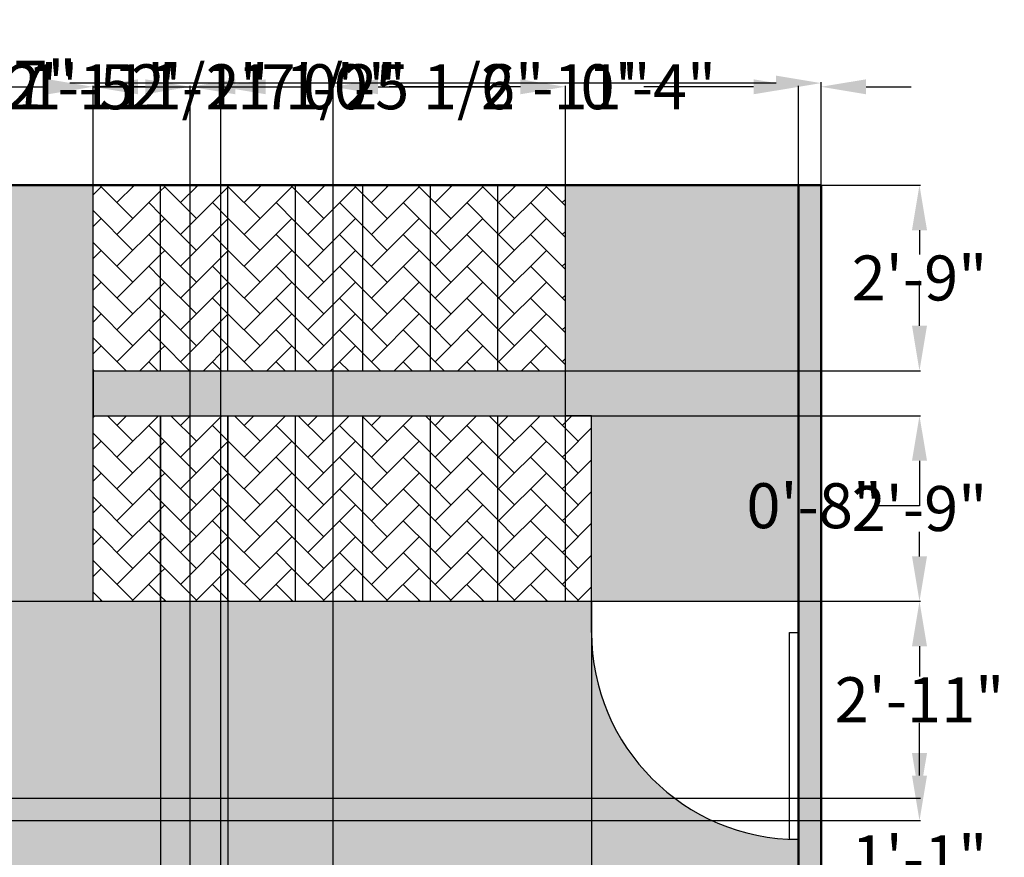
# Model space of a CAD drawing. Units: inches. Extents: x 339 to 824, y 73 to 445.
# Tile 5 of 5: x 605 to 780, y 297 to 445. Entities that reach past the tile are written whole.
import ezdxf

# ---------------------------------------------------------------- set-up
doc = ezdxf.new("R2010")
doc.units = ezdxf.units.IN
doc.header["$MEASUREMENT"] = 0
for name, color, linetype, lineweight in [('A-ANNO-DIMS', 2, 'Continuous', 18), ('A-DOOR', 3, 'Continuous', 25), ('A-FLOR-PATT', 8, 'Continuous', 13), ('A-FLOR-STRS', 7, 'Continuous', 25), ('A-FLOR-STRS-PATT', 252, 'Continuous', 13), ('A-WALL', 7, 'Continuous', 50), ('A-WALL-PATT', 1, 'Continuous', 13)]:
    doc.layers.add(name, color=color, linetype=linetype, lineweight=lineweight)
doc.styles.get("Standard").update_dxf_attribs({"font": 'arial.ttf'})
doc.dimstyles.get("Standard").update_dxf_attribs({"dimtxt": 8, "dimasz": 8, "dimexe": 0.18, "dimexo": 0.0625, "dimgap": 0.09, "dimtad": 0, "dimtih": 1, "dimtoh": 1, "dimdec": 0, "dimzin": 0, "dimdsep": 46, "dimlunit": 3, "dimtxsty": 'Standard', "dimcen": 0.09, "dimadec": 0, "dimazin": 0, "dimtfac": 1, "dimtdec": 0, "dimtofl": 0, "dimtmove": 0, "dimatfit": 3, "dimfxl": 1, "dimtolj": 1, "dimtzin": 0, "dimarcsym": 0})

# ---------------------------------------------------------------- blocks, each defined once
blk = doc.blocks.new('*U4')
for p, q in [((-40, 0), (-40, 6)), ((0, 0), (0, 6))]:
    blk.add_line(p, q)
blk.add_lwpolyline([(0, 0), (0, -40), (-1.75, -40), (-1.75, 0)], close=True)
blk.add_arc((0, 0), 40, 180, 270)
blk = doc.blocks.new('*D11')
at = {"layer": 'A-ANNO-DIMS', "color": 0, "lineweight": -2, "transparency": 16777216}
for p, q in [((452.48, 416.12), (452.48, 434.39)), ((747.48, 416.12), (747.48, 434.39)), ((460.48, 434.21), (586.08, 434.21)), ((739.48, 434.21), (613.88, 434.21))]:
    blk.add_line(p, q, dxfattribs=at)
at = {"layer": 'A-ANNO-DIMS', "color": 0, "transparency": 16777216}
for points in [[(460.48, 435.54), (460.48, 432.88), (452.48, 434.21)], [(739.48, 435.54), (739.48, 432.88), (747.48, 434.21)]]:
    blk.add_solid(points, dxfattribs=at)
at = {"layer": 'Defpoints', "color": 0, "transparency": 16777216}
for p in [(747.48, 434.21), (452.48, 416.06), (747.48, 416.06)]:
    blk.add_point(p, dxfattribs=at)
at = {"layer": 'A-ANNO-DIMS', "color": 0, "transparency": 16777216, "insert": (599.98, 434.21), "char_height": 8, "attachment_point": 5}
blk.add_mtext('\\A1;24\'-7"', dxfattribs=at)
blk = doc.blocks.new('*D20')
at = {"layer": 'A-ANNO-DIMS', "color": 0, "lineweight": -2, "transparency": 16777216}
for p, q in [((558.32, 290.78), (558.32, 288.42)), ((573.25, 290.78), (573.25, 288.42)), ((550.32, 288.6), (542.32, 288.6)), ((581.25, 288.6), (589.25, 288.6))]:
    blk.add_line(p, q, dxfattribs=at)
at = {"layer": 'A-ANNO-DIMS', "color": 0, "transparency": 16777216}
for points in [[(550.32, 289.94), (550.32, 287.27), (558.32, 288.6)], [(581.25, 289.94), (581.25, 287.27), (573.25, 288.6)]]:
    blk.add_solid(points, dxfattribs=at)
at = {"layer": 'Defpoints', "color": 0, "transparency": 16777216}
for p in [(558.32, 290.84), (573.25, 290.84), (573.25, 288.6)]:
    blk.add_point(p, dxfattribs=at)
at = {"layer": 'A-ANNO-DIMS', "color": 0, "transparency": 16777216, "insert": (618.12, 288.6), "char_height": 8, "attachment_point": 5}
blk.add_mtext('\\A1;BASIN 1\'-3"', dxfattribs=at)
blk = doc.blocks.new('*D38')
at = {"layer": 'A-ANNO-DIMS', "color": 0, "lineweight": -2, "transparency": 16777216}
for p, q in [((592.11, 433.56), (584.11, 433.56)), ((600.11, 213.12), (600.11, 433.74)), ((635.29, 213.12), (635.29, 433.74)), ((643.29, 433.56), (651.29, 433.56))]:
    blk.add_line(p, q, dxfattribs=at)
at = {"layer": 'A-ANNO-DIMS', "color": 0, "transparency": 16777216}
for points in [[(592.11, 434.89), (592.11, 432.23), (600.11, 433.56)], [(643.29, 434.89), (643.29, 432.23), (635.29, 433.56)]]:
    blk.add_solid(points, dxfattribs=at)
at = {"layer": 'Defpoints', "color": 0, "transparency": 16777216}
for p in [(635.29, 433.56), (600.11, 213.06), (635.29, 213.06)]:
    blk.add_point(p, dxfattribs=at)
at = {"layer": 'A-ANNO-DIMS', "color": 0, "transparency": 16777216, "insert": (617.7, 433.56), "char_height": 8, "attachment_point": 5}
blk.add_mtext('\\A1;2\'-11"', dxfattribs=at)
blk = doc.blocks.new('*D39')
at = {"layer": 'A-ANNO-DIMS', "color": 0, "lineweight": -2, "transparency": 16777216}
for p, q in [((706.66, 342), (706.66, 84.38)), ((743.48, 342), (743.48, 84.38)), ((698.66, 84.56), (690.66, 84.56)), ((751.48, 84.56), (759.48, 84.56))]:
    blk.add_line(p, q, dxfattribs=at)
at = {"layer": 'A-ANNO-DIMS', "color": 0, "transparency": 16777216}
for points in [[(698.66, 85.89), (698.66, 83.23), (706.66, 84.56)], [(751.48, 85.89), (751.48, 83.23), (743.48, 84.56)]]:
    blk.add_solid(points, dxfattribs=at)
at = {"layer": 'Defpoints', "color": 0, "transparency": 16777216}
for p in [(706.66, 342.06), (743.48, 342.06), (743.48, 84.56)]:
    blk.add_point(p, dxfattribs=at)
at = {"layer": 'A-ANNO-DIMS', "color": 0, "transparency": 16777216, "insert": (725.07, 84.56), "char_height": 8, "attachment_point": 5}
blk.add_mtext('\\A1;3\'-1"', dxfattribs=at)
blk = doc.blocks.new('*D41')
at = {"layer": 'A-ANNO-DIMS', "color": 0, "lineweight": -2, "transparency": 16777216}
for p, q in [((582.55, 342.06), (765.16, 342.06)), ((764.98, 334.06), (764.98, 328.67)), ((764.98, 315.06), (764.98, 320.45)), ((582.55, 307.06), (765.16, 307.06))]:
    blk.add_line(p, q, dxfattribs=at)
at = {"layer": 'A-ANNO-DIMS', "color": 0, "transparency": 16777216}
for points in [[(763.65, 334.06), (766.32, 334.06), (764.98, 342.06)], [(763.65, 315.06), (766.32, 315.06), (764.98, 307.06)]]:
    blk.add_solid(points, dxfattribs=at)
at = {"layer": 'Defpoints', "color": 0, "transparency": 16777216}
for p in [(582.48, 342.06), (582.48, 307.06), (764.98, 307.06)]:
    blk.add_point(p, dxfattribs=at)
at = {"layer": 'A-ANNO-DIMS', "color": 0, "transparency": 16777216, "insert": (764.98, 324.56), "char_height": 8, "attachment_point": 5}
blk.add_mtext('\\A1;2\'-11"', dxfattribs=at)
blk = doc.blocks.new('*D46')
at = {"layer": 'A-ANNO-DIMS', "color": 0, "lineweight": -2, "transparency": 16777216}
for p, q in [((764.98, 311.06), (764.98, 319.06)), ((578.55, 303.06), (765.16, 303.06)), ((578.55, 289.86), (765.16, 289.86)), ((764.98, 281.86), (764.98, 273.86))]:
    blk.add_line(p, q, dxfattribs=at)
at = {"layer": 'A-ANNO-DIMS', "color": 0, "transparency": 16777216}
for points in [[(763.65, 311.06), (766.32, 311.06), (764.98, 303.06)], [(763.65, 281.86), (766.32, 281.86), (764.98, 289.86)]]:
    blk.add_solid(points, dxfattribs=at)
at = {"layer": 'Defpoints', "color": 0, "transparency": 16777216}
for p in [(578.48, 303.06), (578.48, 289.86), (764.98, 289.86)]:
    blk.add_point(p, dxfattribs=at)
at = {"layer": 'A-ANNO-DIMS', "color": 0, "transparency": 16777216, "insert": (764.98, 296.46), "char_height": 8, "attachment_point": 5}
blk.add_mtext('\\A1;1\'-1"', dxfattribs=at)
blk = doc.blocks.new('*D49')
at = {"layer": 'A-ANNO-DIMS', "color": 0, "lineweight": -2, "transparency": 16777216}
for p, q in [((618, 416.12), (618, 433.74)), ((626, 433.56), (649.31, 433.56)), ((694, 433.56), (670.69, 433.56)), ((702, 416.12), (702, 433.74))]:
    blk.add_line(p, q, dxfattribs=at)
at = {"layer": 'A-ANNO-DIMS', "color": 0, "transparency": 16777216}
for points in [[(626, 434.89), (626, 432.23), (618, 433.56)], [(694, 434.89), (694, 432.23), (702, 433.56)]]:
    blk.add_solid(points, dxfattribs=at)
at = {"layer": 'Defpoints', "color": 0, "transparency": 16777216}
for p in [(702, 433.56), (618, 416.06), (702, 416.06)]:
    blk.add_point(p, dxfattribs=at)
at = {"layer": 'A-ANNO-DIMS', "color": 0, "transparency": 16777216, "insert": (660, 433.56), "char_height": 8, "attachment_point": 5}
blk.add_mtext('\\A1;7\'-0"', dxfattribs=at)
blk = doc.blocks.new('*D50')
at = {"layer": 'A-ANNO-DIMS', "color": 0, "lineweight": -2, "transparency": 16777216}
for p, q in [((618.07, 416.06), (765.16, 416.06)), ((764.98, 408.06), (764.98, 403.73)), ((764.98, 391.06), (764.98, 395.39)), ((618.07, 383.06), (765.16, 383.06))]:
    blk.add_line(p, q, dxfattribs=at)
at = {"layer": 'A-ANNO-DIMS', "color": 0, "transparency": 16777216}
for points in [[(763.65, 408.06), (766.32, 408.06), (764.98, 416.06)], [(763.65, 391.06), (766.32, 391.06), (764.98, 383.06)]]:
    blk.add_solid(points, dxfattribs=at)
at = {"layer": 'Defpoints', "color": 0, "transparency": 16777216}
for p in [(618, 416.06), (618, 383.06), (764.98, 383.06)]:
    blk.add_point(p, dxfattribs=at)
at = {"layer": 'A-ANNO-DIMS', "color": 0, "transparency": 16777216, "insert": (764.98, 399.56), "char_height": 8, "attachment_point": 5}
blk.add_mtext('\\A1;2\'-9"', dxfattribs=at)
blk = doc.blocks.new('*D51')
at = {"layer": 'A-ANNO-DIMS', "color": 0, "lineweight": -2, "transparency": 16777216}
for p, q in [((702.07, 375.06), (765.16, 375.06)), ((764.98, 367.06), (764.98, 362.73)), ((764.98, 350.06), (764.98, 354.39)), ((702.07, 342.06), (765.16, 342.06))]:
    blk.add_line(p, q, dxfattribs=at)
at = {"layer": 'A-ANNO-DIMS', "color": 0, "transparency": 16777216}
for points in [[(763.65, 367.06), (766.32, 367.06), (764.98, 375.06)], [(763.65, 350.06), (766.32, 350.06), (764.98, 342.06)]]:
    blk.add_solid(points, dxfattribs=at)
at = {"layer": 'Defpoints', "color": 0, "transparency": 16777216}
for p in [(702, 375.06), (702, 342.06), (764.98, 342.06)]:
    blk.add_point(p, dxfattribs=at)
at = {"layer": 'A-ANNO-DIMS', "color": 0, "transparency": 16777216, "insert": (764.98, 358.56), "char_height": 8, "attachment_point": 5}
blk.add_mtext('\\A1;2\'-9"', dxfattribs=at)
blk = doc.blocks.new('*D52')
at = {"layer": 'A-ANNO-DIMS', "color": 0, "lineweight": -2, "transparency": 16777216}
for p, q in [((764.98, 391.06), (764.98, 399.06)), ((702.07, 383.06), (765.16, 383.06)), ((702.07, 375.06), (765.16, 375.06)), ((764.98, 367.06), (764.98, 359.06)), ((764.98, 359.06), (756.98, 359.06))]:
    blk.add_line(p, q, dxfattribs=at)
at = {"layer": 'A-ANNO-DIMS', "color": 0, "transparency": 16777216}
for points in [[(763.65, 391.06), (766.32, 391.06), (764.98, 383.06)], [(763.65, 367.06), (766.32, 367.06), (764.98, 375.06)]]:
    blk.add_solid(points, dxfattribs=at)
at = {"layer": 'Defpoints', "color": 0, "transparency": 16777216}
for p in [(702, 383.06), (702, 375.06), (764.98, 375.06)]:
    blk.add_point(p, dxfattribs=at)
at = {"layer": 'A-ANNO-DIMS', "color": 0, "transparency": 16777216, "insert": (746.26, 359.06), "char_height": 8, "attachment_point": 5}
blk.add_mtext('\\A1;0\'-8"', dxfattribs=at)
blk = doc.blocks.new('*D53')
at = {"layer": 'A-ANNO-DIMS', "color": 0, "lineweight": -2, "transparency": 16777216}
for p, q in [((630, 375), (630, 84.38)), ((642, 375), (642, 84.38)), ((622, 84.56), (614, 84.56)), ((650, 84.56), (658, 84.56))]:
    blk.add_line(p, q, dxfattribs=at)
at = {"layer": 'A-ANNO-DIMS', "color": 0, "transparency": 16777216}
for points in [[(622, 85.89), (622, 83.23), (630, 84.56)], [(650, 85.89), (650, 83.23), (642, 84.56)]]:
    blk.add_solid(points, dxfattribs=at)
at = {"layer": 'Defpoints', "color": 0, "transparency": 16777216}
for p in [(630, 375.06), (642, 375.06), (642, 84.56)]:
    blk.add_point(p, dxfattribs=at)
at = {"layer": 'A-ANNO-DIMS', "color": 0, "transparency": 16777216, "insert": (668.35, 84.56), "char_height": 8, "attachment_point": 5}
blk.add_mtext('\\A1;1\'-0"', dxfattribs=at)
blk = doc.blocks.new('*D54')
at = {"layer": 'A-ANNO-DIMS', "color": 0, "lineweight": -2, "transparency": 16777216}
for p, q in [((582.48, 416.12), (582.48, 433.74)), ((590.48, 433.56), (610, 433.56)), ((618, 416.12), (618, 433.74)), ((618, 433.56), (626, 433.56))]:
    blk.add_line(p, q, dxfattribs=at)
at = {"layer": 'A-ANNO-DIMS', "color": 0, "transparency": 16777216}
for points in [[(590.48, 434.89), (590.48, 432.23), (582.48, 433.56)], [(610, 434.89), (610, 432.23), (618, 433.56)]]:
    blk.add_solid(points, dxfattribs=at)
at = {"layer": 'Defpoints', "color": 0, "transparency": 16777216}
for p in [(618, 433.56), (582.48, 416.06), (618, 416.06)]:
    blk.add_point(p, dxfattribs=at)
at = {"layer": 'A-ANNO-DIMS', "color": 0, "transparency": 16777216, "insert": (649.22, 433.56), "char_height": 8, "attachment_point": 5}
blk.add_mtext('\\A1;2\'-11 1/2"', dxfattribs=at)
blk = doc.blocks.new('*D55')
at = {"layer": 'A-ANNO-DIMS', "color": 0, "lineweight": -2, "transparency": 16777216}
for p, q in [((582.48, 213.12), (582.48, 433.74)), ((590.48, 433.56), (592.11, 433.56)), ((600.11, 213.12), (600.11, 433.74)), ((600.11, 433.56), (608.11, 433.56))]:
    blk.add_line(p, q, dxfattribs=at)
at = {"layer": 'A-ANNO-DIMS', "color": 0, "transparency": 16777216}
for points in [[(590.48, 434.89), (590.48, 432.23), (582.48, 433.56)], [(592.11, 434.89), (592.11, 432.23), (600.11, 433.56)]]:
    blk.add_solid(points, dxfattribs=at)
at = {"layer": 'Defpoints', "color": 0, "transparency": 16777216}
for p in [(600.11, 433.56), (582.48, 213.06), (600.11, 213.06)]:
    blk.add_point(p, dxfattribs=at)
at = {"layer": 'A-ANNO-DIMS', "color": 0, "transparency": 16777216, "insert": (627.78, 433.56), "char_height": 8, "attachment_point": 5}
blk.add_mtext('\\A1;1\'-5 1/2"', dxfattribs=at)
blk = doc.blocks.new('*D57')
at = {"layer": 'A-ANNO-DIMS', "color": 0, "lineweight": -2, "transparency": 16777216}
for p, q in [((660.7, 241.32), (660.7, 433.74)), ((668.7, 433.56), (688.24, 433.56)), ((735.48, 433.56), (715.95, 433.56)), ((743.48, 281.81), (743.48, 433.74))]:
    blk.add_line(p, q, dxfattribs=at)
at = {"layer": 'A-ANNO-DIMS', "color": 0, "transparency": 16777216}
for points in [[(668.7, 434.89), (668.7, 432.23), (660.7, 433.56)], [(735.48, 434.89), (735.48, 432.23), (743.48, 433.56)]]:
    blk.add_solid(points, dxfattribs=at)
at = {"layer": 'Defpoints', "color": 0, "transparency": 16777216}
for p in [(743.48, 433.56), (743.48, 281.75), (660.7, 241.26)]:
    blk.add_point(p, dxfattribs=at)
at = {"layer": 'A-ANNO-DIMS', "color": 0, "transparency": 16777216, "insert": (702.09, 433.56), "char_height": 8, "attachment_point": 5}
blk.add_mtext('\\A1;6\'-11"', dxfattribs=at)
blk = doc.blocks.new('*D60')
at = {"layer": 'A-ANNO-DIMS', "color": 0, "lineweight": -2, "transparency": 16777216}
for p, q in [((735.48, 433.56), (727.48, 433.56)), ((743.48, 416.12), (743.48, 433.74)), ((747.48, 416.12), (747.48, 433.74)), ((755.48, 433.56), (763.48, 433.56))]:
    blk.add_line(p, q, dxfattribs=at)
at = {"layer": 'A-ANNO-DIMS', "color": 0, "transparency": 16777216}
for points in [[(735.48, 434.89), (735.48, 432.23), (743.48, 433.56)], [(755.48, 434.89), (755.48, 432.23), (747.48, 433.56)]]:
    blk.add_solid(points, dxfattribs=at)
at = {"layer": 'Defpoints', "color": 0, "transparency": 16777216}
for p in [(743.48, 433.56), (743.48, 416.06), (747.48, 416.06)]:
    blk.add_point(p, dxfattribs=at)
at = {"layer": 'A-ANNO-DIMS', "color": 0, "transparency": 16777216, "insert": (716.76, 433.56), "char_height": 8, "attachment_point": 5}
blk.add_mtext('\\A1;0\'-4"', dxfattribs=at)
blk = doc.blocks.new('*D63')
at = {"layer": 'A-ANNO-DIMS', "color": 0, "lineweight": -2, "transparency": 16777216}
for p, q in [((627.29, 433.56), (619.29, 433.56)), ((635.29, 213.12), (635.29, 433.74)), ((640.73, 213.12), (640.73, 433.74)), ((648.73, 433.56), (656.73, 433.56))]:
    blk.add_line(p, q, dxfattribs=at)
at = {"layer": 'A-ANNO-DIMS', "color": 0, "transparency": 16777216}
for points in [[(627.29, 434.89), (627.29, 432.23), (635.29, 433.56)], [(648.73, 434.89), (648.73, 432.23), (640.73, 433.56)]]:
    blk.add_solid(points, dxfattribs=at)
at = {"layer": 'Defpoints', "color": 0, "transparency": 16777216}
for p in [(640.73, 433.56), (635.29, 213.06), (640.73, 213.06)]:
    blk.add_point(p, dxfattribs=at)
at = {"layer": 'A-ANNO-DIMS', "color": 0, "transparency": 16777216, "insert": (676.77, 433.56), "char_height": 8, "attachment_point": 5}
blk.add_mtext('\\A1;0\'-5 1/2"', dxfattribs=at)

msp = doc.modelspace()

# ---------------------------------------------------------------- hatches: boundary and pattern name
at = {"layer": 'A-FLOR-PATT'}
h = msp.add_hatch(color=256, dxfattribs=at)
h.dxf.hatch_style = 1
h.paths.add_polyline_path([(661.42, 241.56), (665.51, 241.56, -0.414214), (667.55, 243.6), (678.83, 243.6, -0.414214), (680.87, 241.56, -0.414214), (682.91, 243.6), (696.76, 243.6, -0.414214), (698.8, 241.56, -0.414214), (700.84, 243.6), (714.97, 243.6, -0.412935), (717.02, 241.56, -0.410727), (719.02, 243.61, -0.419077), (716.95, 245.66), (716.95, 259.06, -0.414214), (718.99, 261.11, -0.414214), (716.95, 263.15), (716.95, 274.6, -0.414214), (718.99, 276.64), (718.99, 280.73, -0.414214), (720.01, 281.75), (743.48, 281.75), (743.48, 293.36), (743.48, 299.72), (741.87, 299.72), (741.87, 299.75, -0.401453), (706.66, 336.54), (706.66, 342.06), (582.48, 342.06), (582.48, 307.06), (582.48, 217.06), (635.29, 217.06), (660.4, 217.06), (660.4, 240.53, -0.414214)])
h.paths.add_polyline_path([(639.94, 279.04), (679.09, 279.04), (679.09, 293.92), (639.94, 293.92)], flags=24)
at = {"layer": 'A-FLOR-STRS-PATT'}
h = msp.add_hatch(color=256, dxfattribs=at)
h.dxf.hatch_style = 1
h.paths.add_polyline_path([(582.48, 351.23), (582.48, 342.06), (618, 342.06), (618, 416.06), (582.48, 416.06), (582.48, 407.26)])
h = msp.add_hatch(dxfattribs=at)
h.set_pattern_fill('AR-HBONE', color=256)
h.paths.add_polyline_path([(630, 416.06), (618, 416.06), (618, 383.06), (630, 383.06)])
h = msp.add_hatch(dxfattribs=at)
h.set_pattern_fill('AR-HBONE', color=256)
h.paths.add_polyline_path([(630, 383.06), (642, 383.06), (642, 416.06), (630, 416.06)])
h = msp.add_hatch(dxfattribs=at)
h.set_pattern_fill('AR-HBONE', color=256)
h.paths.add_polyline_path([(654, 383.06), (654, 416.06), (642, 416.06), (642, 383.06)])
h = msp.add_hatch(dxfattribs=at)
h.set_pattern_fill('AR-HBONE', color=256)
h.paths.add_polyline_path([(654, 383.06), (666, 383.06), (666, 416.06), (654, 416.06)])
h = msp.add_hatch(dxfattribs=at)
h.set_pattern_fill('AR-HBONE', color=256)
h.paths.add_polyline_path([(678, 383.06), (678, 416.06), (666, 416.06), (666, 383.06)])
h = msp.add_hatch(dxfattribs=at)
h.set_pattern_fill('AR-HBONE', color=256)
h.paths.add_polyline_path([(690, 416.06), (678, 416.06), (678, 383.06), (690, 383.06)])
h = msp.add_hatch(dxfattribs=at)
h.set_pattern_fill('AR-HBONE', color=256)
h.paths.add_polyline_path([(690, 383.06), (702, 383.06), (702, 416.06), (690, 416.06)])
h = msp.add_hatch(color=256, dxfattribs=at)
h.dxf.hatch_style = 1
h.paths.add_polyline_path([(706.66, 375.06), (706.66, 342.06), (743.48, 342.06), (743.48, 416.06), (702, 416.06), (702, 375.06)])
h = msp.add_hatch(color=256, dxfattribs=at)
h.dxf.hatch_style = 1
h.paths.add_polyline_path([(702, 375.06), (702, 383.06), (618, 383.06), (618, 375.06)])
h = msp.add_hatch(dxfattribs=at)
h.set_pattern_fill('AR-HBONE', color=256)
h.paths.add_polyline_path([(630, 375.06), (618, 375.06), (618, 342.06), (630, 342.06)])
h = msp.add_hatch(dxfattribs=at)
h.set_pattern_fill('AR-HBONE', color=256)
h.paths.add_polyline_path([(642, 375.06), (630, 375.06), (630, 342.06), (642, 342.06)])
h = msp.add_hatch(dxfattribs=at)
h.set_pattern_fill('AR-HBONE', color=256)
h.paths.add_polyline_path([(642, 342.06), (654, 342.06), (654, 375.06), (642, 375.06)])
h = msp.add_hatch(dxfattribs=at)
h.set_pattern_fill('AR-HBONE', color=256)
h.paths.add_polyline_path([(666, 375.06), (654, 375.06), (654, 342.06), (666, 342.06)])
h = msp.add_hatch(dxfattribs=at)
h.set_pattern_fill('AR-HBONE', color=256)
h.paths.add_polyline_path([(678, 375.06), (666, 375.06), (666, 342.06), (678, 342.06)])
h = msp.add_hatch(dxfattribs=at)
h.set_pattern_fill('AR-HBONE', color=256)
h.paths.add_polyline_path([(690, 375.06), (678, 375.06), (678, 342.06), (690, 342.06)])
h = msp.add_hatch(dxfattribs=at)
h.set_pattern_fill('AR-HBONE', color=256)
h.paths.add_polyline_path([(702, 375.06), (690, 375.06), (690, 342.06), (702, 342.06)])
h = msp.add_hatch(dxfattribs=at)
h.set_pattern_fill('AR-HBONE', color=256)
h.paths.add_polyline_path([(706.66, 375.06), (702, 375.06), (702, 342.06), (706.66, 342.06)])
at = {"layer": 'A-WALL-PATT'}
h = msp.add_hatch(color=256, dxfattribs=at)
h.dxf.hatch_style = 1
h.paths.add_polyline_path([(747.48, 416.06), (743.48, 416.06), (743.48, 293.36), (747.48, 293.36)])

# ---------------------------------------------------------------- linework, layer by layer
at = {"layer": 'A-FLOR-STRS'}
for p, q in [((618, 342.06), (618, 416.06)), ((630, 383.06), (630, 416.06)), ((642, 383.06), (642, 416.06)), ((654, 383.06), (654, 416.06)), ((666, 383.06), (666, 416.06)), ((678, 383.06), (678, 416.06)), ((690, 383.06), (690, 416.06)), ((702, 342.06), (702, 416.06)), ((618, 379.06), (618, 383.06)), ((618, 383.06), (702, 383.06)), ((618, 383.06), (618, 375.06)), ((618, 375.06), (702, 375.06)), ((630, 342.06), (630, 375.06)), ((642, 342.06), (642, 375.06)), ((654, 342.06), (654, 375.06)), ((666, 342.06), (666, 375.06)), ((678, 342.06), (678, 375.06)), ((690, 342.06), (690, 375.06)), ((706.66, 375.06), (702, 375.06)), ((706.66, 342.06), (706.66, 375.06)), ((578.48, 342.06), (743.48, 342.06))]:
    msp.add_line(p, q, dxfattribs=at)
at = {"layer": 'A-WALL'}
for p, q in [((452.48, 416.06), (747.48, 416.06)), ((743.48, 416.06), (747.48, 416.06)), ((743.48, 293.36), (743.48, 416.06)), ((747.48, 416.06), (747.48, 293.36))]:
    msp.add_line(p, q, dxfattribs=at)

# ---------------------------------------------------------------- block references
at = {"layer": 'A-DOOR', "xscale": 0.9204763627207604, "yscale": 0.9204763627207604, "zscale": 0.9204763627207604}
msp.add_blockref('*U4', (743.48, 336.54), dxfattribs=at)

# ---------------------------------------------------------------- dimensions: what is measured, and where the dimension line sits
at = {"layer": 'A-ANNO-DIMS'}
for base, p1, p2, override, picture, middle in [((618, 433.56), (582.48, 416.06), (618, 416.06), {"dimdec": 1, "dimlfac": 1, "dimrnd": 0, "dimzin": 1, "dimdsep": 46, "dimlunit": 4, "dimfrac": 2}, '*D54', (649.22, 433.56)), ((600.11, 433.56), (582.48, 213.06), (600.11, 213.06), {"dimdec": 1, "dimlfac": 1, "dimrnd": 0, "dimzin": 1, "dimdsep": 46, "dimlunit": 4, "dimfrac": 2}, '*D55', (627.78, 433.56)), ((640.73, 433.56), (635.29, 213.06), (640.73, 213.06), {"dimdec": 1, "dimlfac": 1, "dimrnd": 0, "dimzin": 1, "dimdsep": 46, "dimlunit": 4, "dimfrac": 2}, '*D63', (676.77, 433.56)), ((747.48, 434.21), (452.48, 416.06), (747.48, 416.06), {"dimclrd": 0, "dimclre": 0, "dimclrt": 0}, '*D11', (599.98, 434.21)), ((635.29, 433.56), (600.11, 213.06), (635.29, 213.06), {"dimdec": 1, "dimlfac": 1, "dimrnd": 0, "dimzin": 1, "dimdsep": 46, "dimlunit": 4, "dimfrac": 2}, '*D38', (617.7, 433.56)), ((702, 433.56), (618, 416.06), (702, 416.06), {"dimdec": 1, "dimlfac": 1, "dimrnd": 0, "dimzin": 1, "dimdsep": 46, "dimlunit": 4, "dimfrac": 2}, '*D49', (660, 433.56)), ((743.48, 433.56), (660.7, 241.26), (743.48, 281.75), {"dimdec": 1, "dimlfac": 1, "dimrnd": 0, "dimzin": 1, "dimdsep": 46, "dimlunit": 4, "dimfrac": 2}, '*D57', (702.09, 433.56)), ((743.48, 433.56), (747.48, 416.06), (743.48, 416.06), {"dimdec": 1, "dimlfac": 1, "dimrnd": 0, "dimzin": 1, "dimdsep": 46, "dimlunit": 4, "dimfrac": 2}, '*D60', (716.76, 433.56)), ((642, 84.56), (630, 375.06), (642, 375.06), {"dimdec": 1, "dimlfac": 1, "dimrnd": 0, "dimzin": 1, "dimdsep": 46, "dimlunit": 4, "dimfrac": 2}, '*D53', (668.35, 84.56)), ((743.48, 84.56), (706.66, 342.06), (743.48, 342.06), {"dimdec": 1, "dimlfac": 1, "dimrnd": 0, "dimzin": 1, "dimdsep": 46, "dimlunit": 4, "dimfrac": 2}, '*D39', (725.07, 84.56))]:
    dim = msp.add_linear_dim(base=base, p1=p1, p2=p2, dimstyle='Standard', override=override, dxfattribs=at)
    dim.commit()
    dim.dimension.update_dxf_attribs({"geometry": picture, "text_midpoint": middle})
for base, p1, p2, picture, middle in [((764.98, 383.06), (618, 416.06), (618, 383.06), '*D50', (764.98, 399.56)), ((764.98, 375.06), (702, 383.06), (702, 375.06), '*D52', (746.26, 359.06)), ((764.98, 342.06), (702, 375.06), (702, 342.06), '*D51', (764.98, 358.56)), ((764.98, 307.06), (582.48, 342.06), (582.48, 307.06), '*D41', (764.98, 324.56)), ((764.98, 289.86), (578.48, 303.06), (578.48, 289.86), '*D46', (764.98, 296.46))]:
    dim = msp.add_linear_dim(base=base, p1=p1, p2=p2, angle=90, dimstyle='Standard', override={"dimdec": 1, "dimlfac": 1, "dimrnd": 0, "dimzin": 1, "dimdsep": 46, "dimlunit": 4, "dimfrac": 2}, dxfattribs=at)
    dim.commit()
    dim.dimension.update_dxf_attribs({"geometry": picture, "text_midpoint": middle})
dim = msp.add_linear_dim(base=(573.25, 288.6), p1=(558.32, 290.84), p2=(573.25, 290.84), text='BASIN <>', dimstyle='Standard', override={"dimdec": 1, "dimlfac": 1, "dimrnd": 0, "dimzin": 1, "dimdsep": 46, "dimlunit": 4, "dimfrac": 2}, dxfattribs=at)
dim.commit()
dim.dimension.update_dxf_attribs({"geometry": '*D20', "text_midpoint": (618.12, 288.6)})

doc.saveas('drawing.dxf')
